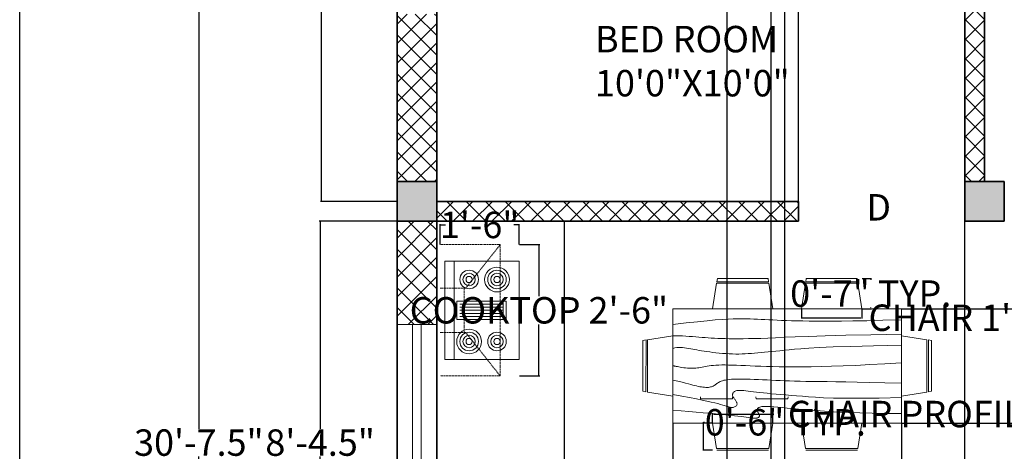
# Model space of a CAD drawing. Units: inches. Extents: x 958 to 1375, y 3152 to 3689.
# Tile 5 of 8: x 958 to 1182, y 3440 to 3538. Entities that reach past the tile are written whole.
import ezdxf

# ---------------------------------------------------------------- set-up
doc = ezdxf.new("R2010")
doc.units = ezdxf.units.IN
doc.header["$MEASUREMENT"] = 0
doc.linetypes.add('HIDDEN2', pattern=[0.1875, 0.125, -0.0625])
for name, color, linetype, lineweight in [('A-ANNO-DIMS', 2, 'Continuous', 18), ('A-ANNO-TTLB', 7, 'Continuous', 25), ('A-AREA-IDEN', 7, 'Continuous', 18), ('A-COLS', 7, 'Continuous', 35), ('A-DOOR-IDEN', 7, 'Continuous', 18), ('A-EQPM', 8, 'Continuous', 18), ('A-EQPM-HIDN', 8, 'HIDDEN2', 13), ('A-FLOR-CASE', 8, 'Continuous', 25), ('A-FURN', 8, 'Continuous', 18), ('A-WALL', 7, 'Continuous', 35), ('windows', 140, 'Continuous', 18)]:
    doc.layers.add(name, color=color, linetype=linetype, lineweight=lineweight)
doc.layers.add('A-COLS-PATT', color=18, linetype='Continuous', lineweight=13, true_color=0x000000)
doc.layers.add('A-WALL-PATT', color=240, linetype='Continuous', lineweight=13, true_color=0xed1f24)
doc.styles.get("Standard").update_dxf_attribs({"font": 'arial.ttf'})
doc.dimstyles.get("Standard").update_dxf_attribs({"dimtxt": 6, "dimasz": 0.18, "dimexe": 0.18, "dimexo": 0.0625, "dimgap": 0.09, "dimtad": 0, "dimtih": 1, "dimtoh": 1, "dimdec": 1, "dimzin": 0, "dimdsep": 46, "dimlunit": 3, "dimtxsty": 'Standard', "dimcen": 0.09, "dimadec": 0, "dimazin": 0, "dimtfac": 1, "dimtdec": 1, "dimtofl": 0, "dimtmove": 0, "dimatfit": 3, "dimfxl": 1, "dimtolj": 1, "dimtzin": 0, "dimarcsym": 0})

# ---------------------------------------------------------------- blocks, each defined once
blk = doc.blocks.new('chimmne')
for points in [[(-13.61, -9.12), (-13.61, 11.28), (13.39, 11.28), (13.39, -9.12)], [(-2.66, -5.87), (-2.66, 7.73), (2.44, 7.73), (2.44, -5.87)]]:
    blk.add_lwpolyline(points, close=True)
for points in [[(-2.66, 6.88), (2.44, 6.88)], [(-1.81, 6.88), (-1.81, -5.02)], [(-0.96, -5.02), (-0.96, 6.88)], [(-0.11, 6.88), (-0.11, -5.02)], [(0.74, -5.02), (0.74, 6.88)], [(1.59, 6.88), (1.59, -5.02)], [(13.39, -6.57), (-13.61, -6.57)]]:
    blk.add_lwpolyline(points)
for centre, radius in [((-8.55, 5.18), 3.4), ((-8.55, 5.18), 2.55), ((-8.55, 5.18), 1.7), ((-8.55, 5.18), 0.85), ((8.44, 5.18), 2.55), ((8.44, 5.18), 1.7), ((8.44, 5.18), 0.85), ((-8.55, -2.47), 2.55), ((8.44, -2.47), 3.4), ((8.44, -2.47), 2.55), ((-8.55, -2.47), 1.7), ((-8.55, -2.47), 0.85), ((8.44, -2.47), 1.7), ((8.44, -2.47), 0.85)]:
    blk.add_circle(centre, radius)
at = {"layer": 'A-EQPM-HIDN'}
for p, q in [((17.89, 6.07), (-18.11, 6.07)), ((-18.11, 6.07), (-18.11, -10.43)), ((-6.16, -3.43), (-18.11, 6.07)), ((5.94, -3.43), (17.89, 6.07)), ((17.89, 6.07), (17.89, -10.43)), ((-6.16, -3.43), (-6.16, -10.43)), ((5.94, -3.82), (-6.16, -3.82)), ((5.94, -3.43), (5.94, -10.43))]:
    blk.add_line(p, q, dxfattribs=at)
blk = doc.blocks.new('*D12')
at = {"layer": 'A-ANNO-DIMS', "color": 0, "lineweight": -2, "transparency": 16777216}
for p, q in [((1044.13, 3616.53), (1026.81, 3616.53)), ((1026.99, 3616.35), (1026.99, 3559.69)), ((1026.99, 3496.71), (1026.99, 3553.38)), ((1044.13, 3496.53), (1026.81, 3496.53))]:
    blk.add_line(p, q, dxfattribs=at)
at = {"layer": 'A-ANNO-DIMS', "color": 0, "transparency": 16777216}
for points in [[(1026.96, 3616.35), (1027.02, 3616.35), (1026.99, 3616.53)], [(1026.96, 3496.71), (1027.02, 3496.71), (1026.99, 3496.53)]]:
    blk.add_solid(points, dxfattribs=at)
at = {"layer": 'Defpoints', "color": 0, "transparency": 16777216}
for p in [(1044.2, 3616.53), (1026.99, 3496.53), (1044.2, 3496.53)]:
    blk.add_point(p, dxfattribs=at)
at = {"layer": 'A-ANNO-DIMS', "color": 0, "transparency": 16777216, "insert": (1026.99, 3556.53), "char_height": 6, "attachment_point": 5}
blk.add_mtext("\\A1;10'", dxfattribs=at)
blk = doc.blocks.new('*D13')
at = {"layer": 'A-ANNO-DIMS', "color": 0, "lineweight": -2, "transparency": 16777216}
for p, q in [((1044.13, 3492.03), (1026.53, 3492.03)), ((1026.71, 3491.85), (1026.71, 3444.94)), ((1026.71, 3391.71), (1026.71, 3438.63)), ((1044.13, 3391.53), (1026.53, 3391.53))]:
    blk.add_line(p, q, dxfattribs=at)
at = {"layer": 'A-ANNO-DIMS', "color": 0, "transparency": 16777216}
for points in [[(1026.68, 3491.85), (1026.74, 3491.85), (1026.71, 3492.03)], [(1026.68, 3391.71), (1026.74, 3391.71), (1026.71, 3391.53)]]:
    blk.add_solid(points, dxfattribs=at)
at = {"layer": 'Defpoints', "color": 0, "transparency": 16777216}
for p in [(1044.2, 3492.03), (1026.71, 3391.53), (1044.2, 3391.53)]:
    blk.add_point(p, dxfattribs=at)
at = {"layer": 'A-ANNO-DIMS', "color": 0, "transparency": 16777216, "insert": (1026.71, 3441.78), "char_height": 6, "attachment_point": 5}
blk.add_mtext('\\A1;8\'-4.5"', dxfattribs=at)
blk = doc.blocks.new('*D15')
at = {"layer": 'A-ANNO-DIMS', "color": 0, "lineweight": -2, "transparency": 16777216}
for p, q in [((1044.13, 3625.53), (998.97, 3625.53)), ((999.15, 3625.35), (999.15, 3444.94)), ((999.15, 3258.21), (999.15, 3438.63)), ((1044.13, 3258.03), (998.97, 3258.03))]:
    blk.add_line(p, q, dxfattribs=at)
at = {"layer": 'A-ANNO-DIMS', "color": 0, "transparency": 16777216}
for points in [[(999.12, 3625.35), (999.18, 3625.35), (999.15, 3625.53)], [(999.12, 3258.21), (999.18, 3258.21), (999.15, 3258.03)]]:
    blk.add_solid(points, dxfattribs=at)
at = {"layer": 'Defpoints', "color": 0, "transparency": 16777216}
for p in [(1044.2, 3625.53), (999.15, 3258.03), (1044.2, 3258.03)]:
    blk.add_point(p, dxfattribs=at)
at = {"layer": 'A-ANNO-DIMS', "color": 0, "transparency": 16777216, "insert": (999.15, 3441.78), "char_height": 6, "attachment_point": 5}
blk.add_mtext('\\A1;30\'-7.5"', dxfattribs=at)
blk = doc.blocks.new('WIN-48')
for p, q in [((48, 9), (0, 9)), ((48, 5.5), (0, 5.5)), ((0, 3.5), (48, 3.5)), ((0, 0), (48, 0))]:
    blk.add_line(p, q)
blk = doc.blocks.new('CHAIR-DINING')
for p, q in [((0.96, 6.13), (1.07, 6.85)), ((12.61, 6.85), (1.07, 6.85)), ((12.61, 6.85), (12.72, 6.13)), ((0, 0), (0.9, 5.77)), ((12.78, 5.77), (0.9, 5.77)), ((0.96, 6.13), (12.72, 6.13)), ((12.78, 5.77), (13.68, 0))]:
    blk.add_line(p, q)
blk = doc.blocks.new('CHAIR-DINING-PROFILE')
for p, q in [((0, 6.13), (0.9, 0.36)), ((12.78, 0.36), (13.68, 6.13)), ((12.78, 0.36), (0.9, 0.36)), ((0.96, 0), (12.72, 0))]:
    blk.add_line(p, q)
blk = doc.blocks.new('*D30')
at = {"layer": 'A-ANNO-DIMS', "color": 0, "lineweight": -2, "transparency": 16777216}
for p, q in [((1136.12, 3472.11), (1136.12, 3469.94)), ((1149.8, 3472.11), (1149.8, 3469.94)), ((1136.3, 3470.12), (1149.62, 3470.12)), ((1149.8, 3470.12), (1149.98, 3470.12))]:
    blk.add_line(p, q, dxfattribs=at)
at = {"layer": 'A-ANNO-DIMS', "color": 0, "transparency": 16777216}
for points in [[(1136.3, 3470.15), (1136.3, 3470.09), (1136.12, 3470.12)], [(1149.62, 3470.15), (1149.62, 3470.09), (1149.8, 3470.12)]]:
    blk.add_solid(points, dxfattribs=at)
at = {"layer": 'Defpoints', "color": 0, "transparency": 16777216}
for p in [(1136.12, 3472.17), (1149.8, 3472.17), (1149.8, 3470.12)]:
    blk.add_point(p, dxfattribs=at)
at = {"layer": 'A-ANNO-DIMS', "color": 0, "transparency": 16777216, "insert": (1189.52, 3470.12), "char_height": 6, "attachment_point": 5}
blk.add_mtext('\\A1;CHAIR 1\'-1 1/2" TYP.', dxfattribs=at)
blk = doc.blocks.new('*D31')
at = {"layer": 'A-ANNO-DIMS', "color": 0, "lineweight": -2, "transparency": 16777216}
for p, q in [((1149.86, 3479.03), (1152.03, 3479.03)), ((1151.85, 3478.85), (1151.85, 3478.75)), ((1149.86, 3472.17), (1152.03, 3472.17)), ((1151.85, 3472.35), (1151.85, 3472.45))]:
    blk.add_line(p, q, dxfattribs=at)
at = {"layer": 'A-ANNO-DIMS', "color": 0, "transparency": 16777216}
for points in [[(1151.82, 3478.85), (1151.88, 3478.85), (1151.85, 3479.03)], [(1151.82, 3472.35), (1151.88, 3472.35), (1151.85, 3472.17)]]:
    blk.add_solid(points, dxfattribs=at)
at = {"layer": 'Defpoints', "color": 0, "transparency": 16777216}
for p in [(1149.8, 3479.03), (1151.85, 3479.03), (1149.8, 3472.17)]:
    blk.add_point(p, dxfattribs=at)
at = {"layer": 'A-ANNO-DIMS', "color": 0, "transparency": 16777216, "insert": (1151.85, 3475.6), "char_height": 6, "attachment_point": 5}
blk.add_mtext('\\A1;0\'-7" TYP.', dxfattribs=at)
blk = doc.blocks.new('*D32')
at = {"layer": 'A-ANNO-DIMS', "color": 0, "lineweight": -2, "transparency": 16777216}
for p, q in [((1115.92, 3446.28), (1115.92, 3448.44)), ((1116.1, 3448.26), (1129.43, 3448.26)), ((1129.61, 3446.28), (1129.61, 3448.44)), ((1129.61, 3448.26), (1129.79, 3448.26))]:
    blk.add_line(p, q, dxfattribs=at)
at = {"layer": 'A-ANNO-DIMS', "color": 0, "transparency": 16777216}
for points in [[(1116.1, 3448.29), (1116.1, 3448.23), (1115.92, 3448.26)], [(1129.43, 3448.29), (1129.43, 3448.23), (1129.61, 3448.26)]]:
    blk.add_solid(points, dxfattribs=at)
at = {"layer": 'Defpoints', "color": 0, "transparency": 16777216}
for p in [(1129.61, 3448.26), (1115.92, 3446.21), (1129.61, 3446.21)]:
    blk.add_point(p, dxfattribs=at)
at = {"layer": 'A-ANNO-DIMS', "color": 0, "transparency": 16777216, "insert": (1188.42, 3448.26), "char_height": 6, "attachment_point": 5}
blk.add_mtext('\\A1;CHAIR PROFILE 1\'-1 1/2" TYP.', dxfattribs=at)
blk = doc.blocks.new('*D33')
at = {"layer": 'A-ANNO-DIMS', "color": 0, "lineweight": -2, "transparency": 16777216}
for p, q in [((1115.86, 3446.21), (1113.69, 3446.21)), ((1113.87, 3446.21), (1113.87, 3446.39)), ((1113.87, 3446.39), (1114.05, 3446.39)), ((1113.87, 3440.26), (1113.87, 3446.03)), ((1115.86, 3440.08), (1113.69, 3440.08))]:
    blk.add_line(p, q, dxfattribs=at)
at = {"layer": 'A-ANNO-DIMS', "color": 0, "transparency": 16777216}
for points in [[(1113.84, 3446.03), (1113.9, 3446.03), (1113.87, 3446.21)], [(1113.84, 3440.26), (1113.9, 3440.26), (1113.87, 3440.08)]]:
    blk.add_solid(points, dxfattribs=at)
at = {"layer": 'Defpoints', "color": 0, "transparency": 16777216}
for p in [(1113.87, 3446.21), (1115.92, 3446.21), (1115.92, 3440.08)]:
    blk.add_point(p, dxfattribs=at)
at = {"layer": 'A-ANNO-DIMS', "color": 0, "transparency": 16777216, "insert": (1132.43, 3446.39), "char_height": 6, "attachment_point": 5}
blk.add_mtext('\\A1;0\'-6" TYP.', dxfattribs=at)
blk = doc.blocks.new('*D34')
at = {"layer": 'A-ANNO-DIMS', "color": 0, "lineweight": -2, "transparency": 16777216}
for p, q in [((1072.02, 3486.71), (1076.61, 3486.71)), ((1076.43, 3486.53), (1076.43, 3475)), ((1076.43, 3457.08), (1076.43, 3468.61)), ((1072.02, 3456.9), (1076.61, 3456.9))]:
    blk.add_line(p, q, dxfattribs=at)
at = {"layer": 'A-ANNO-DIMS', "color": 0, "transparency": 16777216}
for points in [[(1076.4, 3486.53), (1076.46, 3486.53), (1076.43, 3486.71)], [(1076.4, 3457.08), (1076.46, 3457.08), (1076.43, 3456.9)]]:
    blk.add_solid(points, dxfattribs=at)
at = {"layer": 'Defpoints', "color": 0, "transparency": 16777216}
for p in [(1071.96, 3486.71), (1071.96, 3456.9), (1076.43, 3456.9)]:
    blk.add_point(p, dxfattribs=at)
at = {"layer": 'A-ANNO-DIMS', "color": 0, "transparency": 16777216, "insert": (1076.43, 3471.8), "char_height": 6, "attachment_point": 5}
blk.add_mtext('\\A1;COOKTOP 2\'-6"', dxfattribs=at)
blk = doc.blocks.new('*D35')
at = {"layer": 'A-ANNO-DIMS', "color": 0, "lineweight": -2, "transparency": 16777216}
for p, q in [((1053.98, 3486.77), (1053.98, 3491.36)), ((1054.16, 3491.18), (1055.19, 3491.18)), ((1071.78, 3491.18), (1070.75, 3491.18)), ((1071.96, 3486.77), (1071.96, 3491.36))]:
    blk.add_line(p, q, dxfattribs=at)
at = {"layer": 'A-ANNO-DIMS', "color": 0, "transparency": 16777216}
for points in [[(1054.16, 3491.21), (1054.16, 3491.15), (1053.98, 3491.18)], [(1071.78, 3491.21), (1071.78, 3491.15), (1071.96, 3491.18)]]:
    blk.add_solid(points, dxfattribs=at)
at = {"layer": 'Defpoints', "color": 0, "transparency": 16777216}
for p in [(1071.96, 3491.18), (1053.98, 3486.71), (1071.96, 3486.71)]:
    blk.add_point(p, dxfattribs=at)
at = {"layer": 'A-ANNO-DIMS', "color": 0, "transparency": 16777216, "insert": (1062.97, 3491.18), "char_height": 6, "attachment_point": 5}
blk.add_mtext('\\A1;1\'-6"', dxfattribs=at)
blk = doc.blocks.new('*D38')
at = {"layer": 'A-ANNO-DIMS', "color": 0, "lineweight": -2, "transparency": 16777216}
for p, q in [((1106.9, 3446.15), (1106.9, 3234.1)), ((1158.83, 3446.15), (1158.83, 3234.1)), ((1107.08, 3234.28), (1124.68, 3234.28)), ((1158.65, 3234.28), (1141.05, 3234.28))]:
    blk.add_line(p, q, dxfattribs=at)
at = {"layer": 'A-ANNO-DIMS', "color": 0, "transparency": 16777216}
for points in [[(1107.08, 3234.31), (1107.08, 3234.25), (1106.9, 3234.28)], [(1158.65, 3234.31), (1158.65, 3234.25), (1158.83, 3234.28)]]:
    blk.add_solid(points, dxfattribs=at)
at = {"layer": 'Defpoints', "color": 0, "transparency": 16777216}
for p in [(1106.9, 3446.21), (1158.83, 3446.21), (1158.83, 3234.28)]:
    blk.add_point(p, dxfattribs=at)
at = {"layer": 'A-ANNO-DIMS', "color": 0, "transparency": 16777216, "insert": (1132.86, 3234.28), "char_height": 6, "attachment_point": 5}
blk.add_mtext('\\A1;4\'-4"', dxfattribs=at)
blk = doc.blocks.new('*D39')
at = {"layer": 'A-ANNO-DIMS', "color": 0, "lineweight": -2, "transparency": 16777216}
for p, q in [((1158.89, 3472.17), (1330.63, 3472.17)), ((1330.45, 3471.99), (1330.45, 3462.3)), ((1330.45, 3446.39), (1330.45, 3456.09)), ((1158.89, 3446.21), (1330.63, 3446.21))]:
    blk.add_line(p, q, dxfattribs=at)
at = {"layer": 'A-ANNO-DIMS', "color": 0, "transparency": 16777216}
for points in [[(1330.42, 3471.99), (1330.48, 3471.99), (1330.45, 3472.17)], [(1330.42, 3446.39), (1330.48, 3446.39), (1330.45, 3446.21)]]:
    blk.add_solid(points, dxfattribs=at)
at = {"layer": 'Defpoints', "color": 0, "transparency": 16777216}
for p in [(1158.83, 3472.17), (1330.45, 3472.17), (1158.83, 3446.21)]:
    blk.add_point(p, dxfattribs=at)
at = {"layer": 'A-ANNO-DIMS', "color": 0, "transparency": 16777216, "insert": (1330.45, 3459.19), "char_height": 6, "attachment_point": 5}
blk.add_mtext('\\A1;2\'-2"', dxfattribs=at)
blk = doc.blocks.new('*D43')
at = {"layer": 'A-ANNO-DIMS', "color": 0, "lineweight": -2, "transparency": 16777216}
for p, q in [((1119.2, 3303.1), (1119.2, 3649.46)), ((1119.38, 3649.28), (1129.02, 3649.28)), ((1129.2, 3303.1), (1129.2, 3649.46)), ((1129.2, 3649.28), (1129.38, 3649.28))]:
    blk.add_line(p, q, dxfattribs=at)
at = {"layer": 'A-ANNO-DIMS', "color": 0, "transparency": 16777216}
for points in [[(1119.38, 3649.31), (1119.38, 3649.25), (1119.2, 3649.28)], [(1129.02, 3649.31), (1129.02, 3649.25), (1129.2, 3649.28)]]:
    blk.add_solid(points, dxfattribs=at)
at = {"layer": 'Defpoints', "color": 0, "transparency": 16777216}
for p in [(1129.2, 3649.28), (1119.2, 3303.03), (1129.2, 3303.03)]:
    blk.add_point(p, dxfattribs=at)
at = {"layer": 'A-ANNO-DIMS', "color": 0, "transparency": 16777216, "insert": (1139.77, 3649.28), "char_height": 6, "attachment_point": 5}
blk.add_mtext('\\A1;0\'-10"', dxfattribs=at)
blk = doc.blocks.new('*D44')
at = {"layer": 'A-ANNO-DIMS', "color": 0, "lineweight": -2, "transparency": 16777216}
for p, q in [((1132.32, 3267.1), (1132.32, 3649.46)), ((1132.5, 3649.28), (1144.69, 3649.28)), ((1173.02, 3649.28), (1160.82, 3649.28)), ((1173.2, 3267.1), (1173.2, 3649.46))]:
    blk.add_line(p, q, dxfattribs=at)
at = {"layer": 'A-ANNO-DIMS', "color": 0, "transparency": 16777216}
for points in [[(1132.5, 3649.31), (1132.5, 3649.25), (1132.32, 3649.28)], [(1173.02, 3649.31), (1173.02, 3649.25), (1173.2, 3649.28)]]:
    blk.add_solid(points, dxfattribs=at)
at = {"layer": 'Defpoints', "color": 0, "transparency": 16777216}
for p in [(1173.2, 3649.28), (1132.32, 3267.03), (1173.2, 3267.03)]:
    blk.add_point(p, dxfattribs=at)
at = {"layer": 'A-ANNO-DIMS', "color": 0, "transparency": 16777216, "insert": (1152.76, 3649.28), "char_height": 6, "attachment_point": 5}
blk.add_mtext('\\A1;3\'-5"', dxfattribs=at)
blk = doc.blocks.new('*D46')
at = {"layer": 'A-ANNO-DIMS', "color": 0, "lineweight": -2, "transparency": 16777216}
for p, q in [((1135.44, 3496.6), (1135.44, 3649.46)), ((1135.62, 3649.28), (1146.25, 3649.28)), ((1173.02, 3649.28), (1162.38, 3649.28)), ((1173.2, 3492.1), (1173.2, 3649.46))]:
    blk.add_line(p, q, dxfattribs=at)
at = {"layer": 'A-ANNO-DIMS', "color": 0, "transparency": 16777216}
for points in [[(1135.62, 3649.31), (1135.62, 3649.25), (1135.44, 3649.28)], [(1173.02, 3649.31), (1173.02, 3649.25), (1173.2, 3649.28)]]:
    blk.add_solid(points, dxfattribs=at)
at = {"layer": 'Defpoints', "color": 0, "transparency": 16777216}
for p in [(1173.2, 3649.28), (1135.44, 3496.53), (1173.2, 3492.03)]:
    blk.add_point(p, dxfattribs=at)
at = {"layer": 'A-ANNO-DIMS', "color": 0, "transparency": 16777216, "insert": (1154.32, 3649.28), "char_height": 6, "attachment_point": 5}
blk.add_mtext('\\A1;3\'-2"', dxfattribs=at)

msp = doc.modelspace()

# ---------------------------------------------------------------- hatches: boundary and pattern name
at = {"layer": 'A-COLS-PATT'}
h = msp.add_hatch(color=256, dxfattribs=at)
h.dxf.hatch_style = 1
h.paths.add_polyline_path([(1053.2, 3625.53), (1044.2, 3625.53), (1044.2, 3616.53), (1053.2, 3616.53)])
h.paths.add_polyline_path([(1182.2, 3625.53), (1173.2, 3625.53), (1173.2, 3616.53), (1182.2, 3616.53)])
h.paths.add_polyline_path([(1306.7, 3625.53), (1297.7, 3625.53), (1297.7, 3616.53), (1306.7, 3616.53)])
h.paths.add_polyline_path([(1306.7, 3501.03), (1297.7, 3501.03), (1297.7, 3492.03), (1306.7, 3492.03)])
h.paths.add_polyline_path([(1306.7, 3391.53), (1297.7, 3391.53), (1297.7, 3382.53), (1306.7, 3382.53)])
h.paths.add_polyline_path([(1306.7, 3267.03), (1297.7, 3267.03), (1297.7, 3258.03), (1306.7, 3258.03)])
h.paths.add_polyline_path([(1182.2, 3267.03), (1173.2, 3267.03), (1173.2, 3258.03), (1182.2, 3258.03)])
h.paths.add_polyline_path([(1053.2, 3267.03), (1044.2, 3267.03), (1044.2, 3258.03), (1053.2, 3258.03)])
h.paths.add_polyline_path([(1053.2, 3391.53), (1044.2, 3391.53), (1044.2, 3382.53), (1053.2, 3382.53)])
h.paths.add_polyline_path([(1053.2, 3501.03), (1044.2, 3501.03), (1044.2, 3492.03), (1053.2, 3492.03)])
h.paths.add_polyline_path([(1182.2, 3501.03), (1173.2, 3501.03), (1173.2, 3492.03), (1182.2, 3492.03)])
h.paths.add_polyline_path([(1182.2, 3391.53), (1173.2, 3391.53), (1173.2, 3382.53), (1182.2, 3382.53)])
at = {"layer": 'A-WALL-PATT'}
h = msp.add_hatch(dxfattribs=at)
h.set_pattern_fill('ANSI37', color=256, scale=25)
h.paths.add_polyline_path([(1080.68, 3625.53), (1053.2, 3625.53), (1053.2, 3616.53), (1080.68, 3616.53)])
h.paths.add_polyline_path([(1053.2, 3616.53), (1044.2, 3616.53), (1044.2, 3587.05), (1053.2, 3587.05)])
h.paths.add_polyline_path([(1173.2, 3625.53), (1128.68, 3625.53), (1128.68, 3616.53), (1173.2, 3616.53)])
h.paths.add_polyline_path([(1215.78, 3625.53), (1182.2, 3625.53), (1182.2, 3616.53), (1215.78, 3616.53)])
h.paths.add_polyline_path([(1297.7, 3625.53), (1263.78, 3625.53), (1263.78, 3616.53), (1297.7, 3616.53)])
h.paths.add_polyline_path([(1177.7, 3616.53), (1173.2, 3616.53), (1173.2, 3501.03), (1177.7, 3501.03)])
h.paths.add_polyline_path([(1053.2, 3539.05), (1044.2, 3539.05), (1044.2, 3501.03), (1053.2, 3501.03)])
h.paths.add_polyline_path([(1135.44, 3496.53), (1053.2, 3496.53), (1053.2, 3492.03), (1135.44, 3492.03)])
h.paths.add_polyline_path([(1306.7, 3616.53), (1297.7, 3616.53), (1297.7, 3586.38), (1306.7, 3586.38)])
h.paths.add_polyline_path([(1306.7, 3538.38), (1297.7, 3538.38), (1297.7, 3501.03), (1306.7, 3501.03)])
h.paths.add_polyline_path([(1297.7, 3496.53), (1216.84, 3496.53), (1216.84, 3492.03), (1297.7, 3492.03)])
h.paths.add_polyline_path([(1306.7, 3492.03), (1297.7, 3492.03), (1297.7, 3481.63), (1306.7, 3481.63)])
h.paths.add_polyline_path([(1306.7, 3457.63), (1297.7, 3457.63), (1297.7, 3444.03), (1225.7, 3444.03), (1225.7, 3462.51), (1221.2, 3462.51), (1221.2, 3391.53), (1182.2, 3391.53), (1182.2, 3387.03), (1225.7, 3387.03), (1225.7, 3439.53), (1297.7, 3439.53), (1297.7, 3428.57), (1306.7, 3428.57)])
h.paths.add_polyline_path([(1306.7, 3404.57), (1297.7, 3404.57), (1297.7, 3391.53), (1306.7, 3391.53)], flags=17)
h.paths.add_polyline_path([(1297.7, 3391.53), (1253.12, 3391.53), (1253.12, 3387.03), (1297.7, 3387.03)], flags=17)
h.paths.add_polyline_path([(1306.7, 3382.53), (1297.7, 3382.53), (1297.7, 3354.01), (1306.7, 3354.01)])
h.paths.add_polyline_path([(1306.7, 3306.01), (1297.7, 3306.01), (1297.7, 3267.03), (1306.7, 3267.03)])
h.paths.add_polyline_path([(1297.7, 3267.03), (1254.05, 3267.03), (1254.05, 3258.03), (1297.7, 3258.03)])
h.paths.add_polyline_path([(1177.7, 3347.74), (1173.2, 3347.74), (1173.2, 3267.03), (1177.7, 3267.03)])
h.paths.add_polyline_path([(1206.05, 3267.03), (1182.2, 3267.03), (1182.2, 3258.03), (1206.05, 3258.03)])
h.paths.add_polyline_path([(1053.2, 3308.96), (1044.2, 3308.96), (1044.2, 3267.03), (1053.2, 3267.03)])
h.paths.add_polyline_path([(1053.2, 3382.53), (1044.2, 3382.53), (1044.2, 3356.96), (1053.2, 3356.96)])
h.paths.add_polyline_path([(1053.2, 3420.58), (1044.2, 3420.58), (1044.2, 3391.53), (1053.2, 3391.53)])
h.paths.add_polyline_path([(1053.2, 3492.03), (1044.2, 3492.03), (1044.2, 3468.58), (1053.2, 3468.58)])

# ---------------------------------------------------------------- linework, layer by layer
at = {"layer": 'A-ANNO-TTLB'}
msp.add_lwpolyline([(958.44, 3689.37), (1374.91, 3689.37), (1374.91, 3152.28), (958.44, 3152.28)], close=True, dxfattribs=at)
at = {"layer": 'A-COLS'}
for p, q in [((1044.2, 3492.03), (1044.2, 3501.03)), ((1044.2, 3501.03), (1053.2, 3501.03)), ((1053.2, 3501.03), (1053.2, 3492.03)), ((1173.2, 3492.03), (1173.2, 3501.03)), ((1173.2, 3501.03), (1182.2, 3501.03)), ((1182.2, 3501.03), (1182.2, 3492.03)), ((1044.2, 3492.03), (1044.2, 3492.03)), ((1182.2, 3492.03), (1173.2, 3492.03)), ((1173.2, 3492.03), (1173.2, 3492.03))]:
    msp.add_line(p, q, dxfattribs=at)
at = {"layer": 'A-FLOR-CASE'}
msp.add_line((1082.2, 3492.03), (1082.2, 3391.53), dxfattribs=at)
at = {"layer": 'A-FURN'}
for p, q in [((1158.83, 3472.17), (1106.9, 3472.17)), ((1106.9, 3472.17), (1106.9, 3446.21)), ((1158.83, 3446.21), (1158.83, 3472.17)), ((1113.12, 3452.17), (1113.19, 3451.72)), ((1120.39, 3451.72), (1113.19, 3451.72)), ((1120.39, 3451.72), (1120.46, 3452.17)), ((1125.71, 3452.17), (1125.78, 3451.72)), ((1132.98, 3451.72), (1125.78, 3451.72)), ((1132.98, 3451.72), (1133.05, 3452.17)), ((1106.9, 3446.21), (1158.83, 3446.21))]:
    msp.add_line(p, q, dxfattribs=at)
for points in [[(1158.83, 3469.65), (1154.56, 3469.53), (1150.92, 3469.44), (1147.81, 3469.38), (1145.18, 3469.34), (1142.94, 3469.32), (1141.01, 3469.32), (1139.33, 3469.33), (1137.82, 3469.35), (1136.41, 3469.38), (1135.09, 3469.41), (1133.85, 3469.44), (1132.69, 3469.48), (1131.59, 3469.52), (1130.56, 3469.56), (1129.58, 3469.61), (1128.66, 3469.65), (1127.77, 3469.7), (1126.92, 3469.74), (1126.09, 3469.78), (1125.26, 3469.81), (1124.41, 3469.84), (1123.54, 3469.86), (1122.62, 3469.87), (1121.65, 3469.86), (1120.61, 3469.84), (1119.44, 3469.8), (1118.09, 3469.72), (1116.52, 3469.61), (1114.66, 3469.45), (1112.48, 3469.22), (1109.91, 3468.93), (1106.9, 3468.57)], [(1158.83, 3466.41), (1151.9, 3466.27), (1146.18, 3466.14), (1141.51, 3466.01), (1137.72, 3465.89), (1134.68, 3465.77), (1132.23, 3465.67), (1130.21, 3465.58), (1128.47, 3465.5), (1126.89, 3465.44), (1125.43, 3465.4), (1124.08, 3465.37), (1122.84, 3465.35), (1121.69, 3465.35), (1120.63, 3465.35), (1119.65, 3465.36), (1118.74, 3465.38), (1117.89, 3465.41), (1117.09, 3465.44), (1116.33, 3465.47), (1115.61, 3465.51), (1114.9, 3465.56), (1114.2, 3465.61), (1113.5, 3465.66), (1112.79, 3465.71), (1112.06, 3465.77), (1111.31, 3465.83), (1110.55, 3465.88), (1109.8, 3465.94), (1109.05, 3465.98), (1108.31, 3466.01), (1107.59, 3466.04), (1106.9, 3466.04)], [(1158.83, 3463.88), (1152.47, 3463.75), (1147.35, 3463.61), (1143.3, 3463.48), (1140.15, 3463.35), (1137.75, 3463.22), (1135.92, 3463.09), (1134.49, 3462.97), (1133.31, 3462.86), (1132.23, 3462.75), (1131.22, 3462.64), (1130.27, 3462.55), (1129.38, 3462.45), (1128.53, 3462.37), (1127.72, 3462.28), (1126.94, 3462.21), (1126.19, 3462.14), (1125.45, 3462.07), (1124.73, 3462.02), (1124.02, 3461.97), (1123.31, 3461.93), (1122.6, 3461.9), (1121.88, 3461.88), (1121.16, 3461.88), (1120.42, 3461.9), (1119.67, 3461.93), (1118.91, 3461.97), (1118.15, 3462.03), (1117.39, 3462.1), (1116.65, 3462.18), (1115.93, 3462.26), (1115.24, 3462.35), (1114.59, 3462.44), (1113.98, 3462.53), (1113.41, 3462.62), (1112.87, 3462.71), (1112.36, 3462.8), (1111.87, 3462.88), (1111.4, 3462.97), (1110.94, 3463.05), (1110.47, 3463.13), (1110.01, 3463.21), (1109.55, 3463.27), (1109.09, 3463.33), (1108.63, 3463.36), (1108.18, 3463.36), (1107.74, 3463.34), (1107.31, 3463.27), (1106.9, 3463.16)], [(1158.83, 3459.91), (1155.07, 3459.67), (1151.63, 3459.47), (1148.48, 3459.31), (1145.6, 3459.19), (1142.96, 3459.1), (1140.54, 3459.04), (1138.33, 3459), (1136.29, 3458.98), (1134.4, 3458.98), (1132.65, 3458.99), (1131.04, 3459), (1129.53, 3459.03), (1128.14, 3459.07), (1126.83, 3459.11), (1125.6, 3459.15), (1124.45, 3459.19), (1123.35, 3459.24), (1122.31, 3459.28), (1121.32, 3459.32), (1120.4, 3459.35), (1119.53, 3459.37), (1118.73, 3459.39), (1117.98, 3459.39), (1117.3, 3459.37), (1116.67, 3459.34), (1116.1, 3459.3), (1115.59, 3459.24), (1115.11, 3459.18), (1114.67, 3459.11), (1114.26, 3459.04), (1113.88, 3458.96), (1113.51, 3458.89), (1113.15, 3458.83), (1112.8, 3458.77), (1112.46, 3458.72), (1112.11, 3458.68), (1111.76, 3458.65), (1111.4, 3458.64), (1111.02, 3458.64), (1110.62, 3458.65), (1110.21, 3458.68), (1109.78, 3458.73), (1109.36, 3458.78), (1108.95, 3458.84), (1108.56, 3458.9), (1108.2, 3458.96), (1107.9, 3459.02), (1107.65, 3459.07), (1107.47, 3459.11), (1107.34, 3459.14), (1107.26, 3459.16), (1107.19, 3459.18), (1107.14, 3459.19), (1107.09, 3459.19), (1107.01, 3459.19), (1106.9, 3459.19)], [(1158.83, 3455.23), (1155.02, 3455.35), (1151.66, 3455.44), (1148.73, 3455.5), (1146.15, 3455.55), (1143.9, 3455.58), (1141.91, 3455.61), (1140.15, 3455.63), (1138.57, 3455.65), (1137.12, 3455.67), (1135.79, 3455.7), (1134.55, 3455.74), (1133.4, 3455.77), (1132.3, 3455.82), (1131.26, 3455.86), (1130.25, 3455.9), (1129.26, 3455.95), (1128.27, 3455.99), (1127.28, 3456.04), (1126.32, 3456.08), (1125.38, 3456.11), (1124.47, 3456.14), (1123.61, 3456.17), (1122.8, 3456.18), (1122.04, 3456.19), (1121.36, 3456.18), (1120.73, 3456.17), (1120.17, 3456.14), (1119.66, 3456.1), (1119.21, 3456.05), (1118.81, 3455.98), (1118.45, 3455.91), (1118.14, 3455.83), (1117.86, 3455.73), (1117.62, 3455.63), (1117.41, 3455.52), (1117.22, 3455.4), (1117.05, 3455.28), (1116.89, 3455.16), (1116.73, 3455.04), (1116.57, 3454.93), (1116.41, 3454.82), (1116.24, 3454.71), (1116.07, 3454.62), (1115.88, 3454.53), (1115.67, 3454.46), (1115.45, 3454.4), (1115.21, 3454.36), (1114.95, 3454.32), (1114.67, 3454.31), (1114.37, 3454.31), (1114.05, 3454.33), (1113.71, 3454.36), (1113.36, 3454.41), (1113, 3454.47), (1112.63, 3454.54), (1112.25, 3454.63), (1111.86, 3454.72), (1111.44, 3454.83), (1110.96, 3454.96), (1110.41, 3455.11), (1109.75, 3455.28), (1108.96, 3455.47), (1108.02, 3455.69), (1106.9, 3455.95)], [(1158.83, 3451.98), (1153.76, 3451.88), (1149.57, 3451.83), (1146.15, 3451.84), (1143.37, 3451.88), (1141.11, 3451.96), (1139.26, 3452.06), (1137.71, 3452.17), (1136.32, 3452.28), (1135, 3452.39), (1133.75, 3452.5), (1132.54, 3452.6), (1131.4, 3452.69), (1130.32, 3452.79), (1129.3, 3452.88), (1128.34, 3452.97), (1127.45, 3453.06), (1126.63, 3453.15), (1125.87, 3453.24), (1125.18, 3453.32), (1124.55, 3453.4), (1123.97, 3453.47), (1123.46, 3453.53), (1122.99, 3453.57), (1122.58, 3453.6), (1122.23, 3453.62), (1121.91, 3453.62), (1121.64, 3453.6), (1121.41, 3453.57), (1121.21, 3453.52), (1121.05, 3453.46), (1120.9, 3453.39), (1120.78, 3453.3), (1120.68, 3453.21), (1120.59, 3453.1), (1120.52, 3452.99), (1120.47, 3452.87), (1120.44, 3452.74), (1120.44, 3452.61), (1120.45, 3452.48), (1120.48, 3452.34), (1120.54, 3452.21), (1120.61, 3452.07), (1120.7, 3451.94), (1120.8, 3451.8), (1120.9, 3451.67), (1121.01, 3451.53), (1121.11, 3451.39), (1121.2, 3451.26), (1121.29, 3451.12), (1121.36, 3450.99), (1121.41, 3450.86), (1121.45, 3450.73), (1121.47, 3450.6), (1121.46, 3450.47), (1121.44, 3450.35), (1121.38, 3450.24), (1121.3, 3450.13), (1121.19, 3450.03), (1121.06, 3449.94), (1120.91, 3449.86), (1120.74, 3449.8), (1120.55, 3449.76), (1120.34, 3449.75), (1120.12, 3449.76), (1119.89, 3449.79), (1119.63, 3449.85), (1119.35, 3449.94), (1119.02, 3450.05), (1118.64, 3450.17), (1118.2, 3450.31), (1117.68, 3450.46), (1117.09, 3450.63), (1116.39, 3450.8), (1115.58, 3450.99), (1114.63, 3451.2), (1113.51, 3451.43), (1112.21, 3451.69), (1110.68, 3451.98), (1108.92, 3452.32), (1106.9, 3452.7)], [(1158.83, 3448.37), (1155.35, 3448.39), (1152.2, 3448.44), (1149.34, 3448.51), (1146.76, 3448.6), (1144.43, 3448.71), (1142.31, 3448.83), (1140.37, 3448.96), (1138.6, 3449.1), (1136.97, 3449.23), (1135.46, 3449.36), (1134.08, 3449.49), (1132.84, 3449.61), (1131.71, 3449.71), (1130.71, 3449.81), (1129.83, 3449.88), (1129.08, 3449.94), (1128.43, 3449.97), (1127.9, 3449.98), (1127.46, 3449.98), (1127.11, 3449.95), (1126.83, 3449.91), (1126.61, 3449.85), (1126.44, 3449.78), (1126.31, 3449.7), (1126.21, 3449.6), (1126.14, 3449.5), (1126.09, 3449.39), (1126.06, 3449.27), (1126.06, 3449.15), (1126.07, 3449.03), (1126.09, 3448.91), (1126.13, 3448.8), (1126.18, 3448.69), (1126.24, 3448.58), (1126.3, 3448.48), (1126.36, 3448.38), (1126.42, 3448.29), (1126.48, 3448.2), (1126.52, 3448.1), (1126.55, 3448.01), (1126.57, 3447.92), (1126.56, 3447.84), (1126.54, 3447.75), (1126.51, 3447.67), (1126.45, 3447.59), (1126.38, 3447.52), (1126.3, 3447.46), (1126.19, 3447.41), (1126.07, 3447.37), (1125.93, 3447.35), (1125.76, 3447.33), (1125.56, 3447.32), (1125.33, 3447.33), (1125.06, 3447.35), (1124.75, 3447.37), (1124.39, 3447.41), (1123.98, 3447.46), (1123.51, 3447.52), (1122.97, 3447.6), (1122.36, 3447.68), (1121.65, 3447.76), (1120.86, 3447.86), (1119.96, 3447.96), (1118.95, 3448.07), (1117.82, 3448.19), (1116.57, 3448.31), (1115.21, 3448.43), (1113.75, 3448.56), (1112.18, 3448.69), (1110.51, 3448.83), (1108.75, 3448.96), (1106.9, 3449.1)]]:
    msp.add_lwpolyline(points, dxfattribs=at)
at = {"layer": 'A-WALL'}
for p, q in [((1044.2, 3625.53), (1044.2, 3258.03)), ((1053.2, 3625.53), (1053.2, 3258.03)), ((1173.2, 3625.53), (1173.2, 3492.03)), ((1173.2, 3625.53), (1173.2, 3492.03)), ((1177.7, 3616.53), (1177.7, 3501.03)), ((1177.7, 3616.53), (1177.7, 3501.03)), ((1053.2, 3496.53), (1135.44, 3496.53)), ((1135.44, 3496.53), (1135.44, 3492.03)), ((1044.2, 3492.03), (1135.44, 3492.03)), ((1173.2, 3492.03), (1177.7, 3492.03))]:
    msp.add_line(p, q, dxfattribs=at)
at = {"layer": 'windows'}
msp.add_line((1044.2, 3468.58), (1053.2, 3468.58), dxfattribs=at)

# ---------------------------------------------------------------- block references
at = {"layer": 'A-EQPM', "xscale": 0.8280321260258986, "yscale": 0.8280321260258986, "zscale": 0.8280321260258986, "rotation": 270}
msp.add_blockref('chimmne', (1062.62, 3471.71), dxfattribs=at)
at = {"layer": 'A-FURN'}
for name, p in [('CHAIR-DINING', (1115.92, 3472.17)), ('CHAIR-DINING', (1136.12, 3472.17)), ('CHAIR-DINING-PROFILE', (1115.92, 3440.08)), ('CHAIR-DINING-PROFILE', (1136.12, 3440.08))]:
    msp.add_blockref(name, p, dxfattribs=at)
for p, rotation in [((1106.9, 3452.35), 89.99413959734413), ((1158.82, 3466.03), 270.0000441631949)]:
    msp.add_blockref('CHAIR-DINING', p, dxfattribs=dict(at, rotation=rotation))
at = {"layer": 'windows', "rotation": 90}
msp.add_blockref('WIN-48', (1053.2, 3420.58), dxfattribs=at)

# ---------------------------------------------------------------- texts
at = {"layer": 'A-AREA-IDEN', "insert": (1089.17, 3536.35), "char_height": 6, "attachment_point": 1}
msp.add_mtext_dynamic_manual_height_columns('BED ROOM\\P10\'0"X10\'0"', width=148.5008, gutter_width=1, heights=[0], dxfattribs=at)
at = {"layer": 'A-DOOR-IDEN', "insert": (1150.82, 3498.18), "char_height": 6, "attachment_point": 1}
msp.add_mtext_dynamic_manual_height_columns('D ', width=17.9455, gutter_width=1, heights=[0], dxfattribs=at)

# ---------------------------------------------------------------- dimensions: what is measured, and where the dimension line sits
at = {"layer": 'A-ANNO-DIMS'}
for base, p1, p2, picture, middle in [((1129.2, 3649.28), (1119.2, 3303.03), (1129.2, 3303.03), '*D43', (1139.77, 3649.28)), ((1173.2, 3649.28), (1132.32, 3267.03), (1173.2, 3267.03), '*D44', (1152.76, 3649.28)), ((1173.2, 3649.28), (1135.44, 3496.53), (1173.2, 3492.03), '*D46', (1154.32, 3649.28)), ((1071.96, 3491.18), (1053.98, 3486.71), (1071.96, 3486.71), '*D35', (1062.97, 3491.18)), ((1158.83, 3234.28), (1106.9, 3446.21), (1158.83, 3446.21), '*D38', (1132.86, 3234.28))]:
    dim = msp.add_linear_dim(base=base, p1=p1, p2=p2, dimstyle='Standard', override={"dimdec": 1, "dimlfac": 1, "dimrnd": 0, "dimzin": 1, "dimdsep": 46, "dimlunit": 4, "dimfrac": 2}, dxfattribs=at)
    dim.commit()
    dim.dimension.update_dxf_attribs({"geometry": picture, "text_midpoint": middle})
for base, p1, p2, override, picture, middle in [((999.15, 3258.03), (1044.2, 3625.53), (1044.2, 3258.03), {"dimclrd": 0, "dimclre": 0, "dimclrt": 0}, '*D15', (999.15, 3441.78)), ((1026.99, 3496.53), (1044.2, 3616.53), (1044.2, 3496.53), {"dimclrd": 0, "dimclre": 0, "dimclrt": 0}, '*D12', (1026.99, 3556.53)), ((1026.71, 3391.53), (1044.2, 3492.03), (1044.2, 3391.53), {"dimclrd": 0, "dimclre": 0, "dimclrt": 0}, '*D13', (1026.71, 3441.78)), ((1330.45, 3472.17), (1158.83, 3446.21), (1158.83, 3472.17), {"dimdec": 1, "dimlfac": 1, "dimrnd": 0, "dimzin": 1, "dimdsep": 46, "dimlunit": 4, "dimfrac": 2}, '*D39', (1330.45, 3459.19))]:
    dim = msp.add_linear_dim(base=base, p1=p1, p2=p2, angle=90, dimstyle='Standard', override=override, dxfattribs=at)
    dim.commit()
    dim.dimension.update_dxf_attribs({"geometry": picture, "text_midpoint": middle})
for base, p1, p2, text, picture, middle in [((1149.8, 3470.12), (1136.12, 3472.17), (1149.8, 3472.17), 'CHAIR <> TYP.', '*D30', (1189.52, 3470.12)), ((1129.61, 3448.26), (1115.92, 3446.21), (1129.61, 3446.21), 'CHAIR PROFILE <> TYP.', '*D32', (1188.42, 3448.26))]:
    dim = msp.add_linear_dim(base=base, p1=p1, p2=p2, text=text, dimstyle='Standard', override={"dimdec": 1, "dimlfac": 1, "dimrnd": 0, "dimzin": 1, "dimdsep": 46, "dimlunit": 4, "dimfrac": 2}, dxfattribs=at)
    dim.commit()
    dim.dimension.update_dxf_attribs({"geometry": picture, "text_midpoint": middle})
for base, p1, p2, angle, text, picture, middle in [((1076.43, 3456.9), (1071.96, 3486.71), (1071.96, 3456.9), 270, 'COOKTOP <>', '*D34', (1076.43, 3471.8)), ((1151.85, 3479.03), (1149.8, 3472.17), (1149.8, 3479.03), 90, '<> TYP.', '*D31', (1151.85, 3475.6)), ((1113.87, 3446.21), (1115.92, 3440.08), (1115.92, 3446.21), 90, '<> TYP.', '*D33', (1132.43, 3446.39))]:
    dim = msp.add_linear_dim(base=base, p1=p1, p2=p2, angle=angle, text=text, dimstyle='Standard', override={"dimdec": 1, "dimlfac": 1, "dimrnd": 0, "dimzin": 1, "dimdsep": 46, "dimlunit": 4, "dimfrac": 2}, dxfattribs=at)
    dim.commit()
    dim.dimension.update_dxf_attribs({"geometry": picture, "text_midpoint": middle})

doc.saveas('drawing.dxf')
